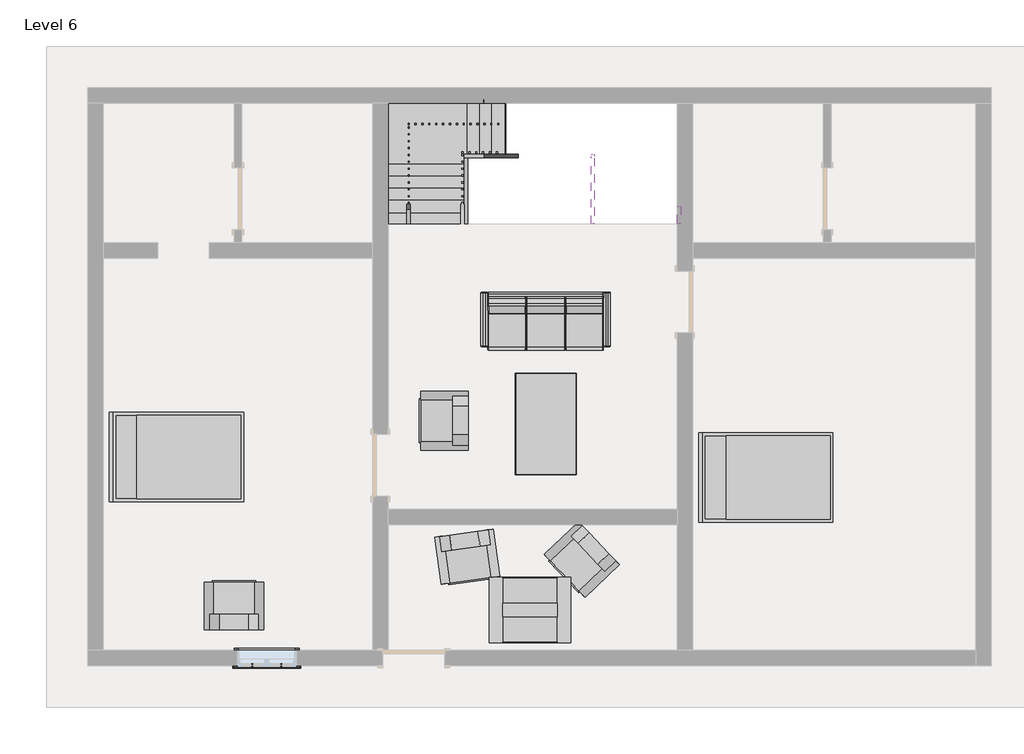
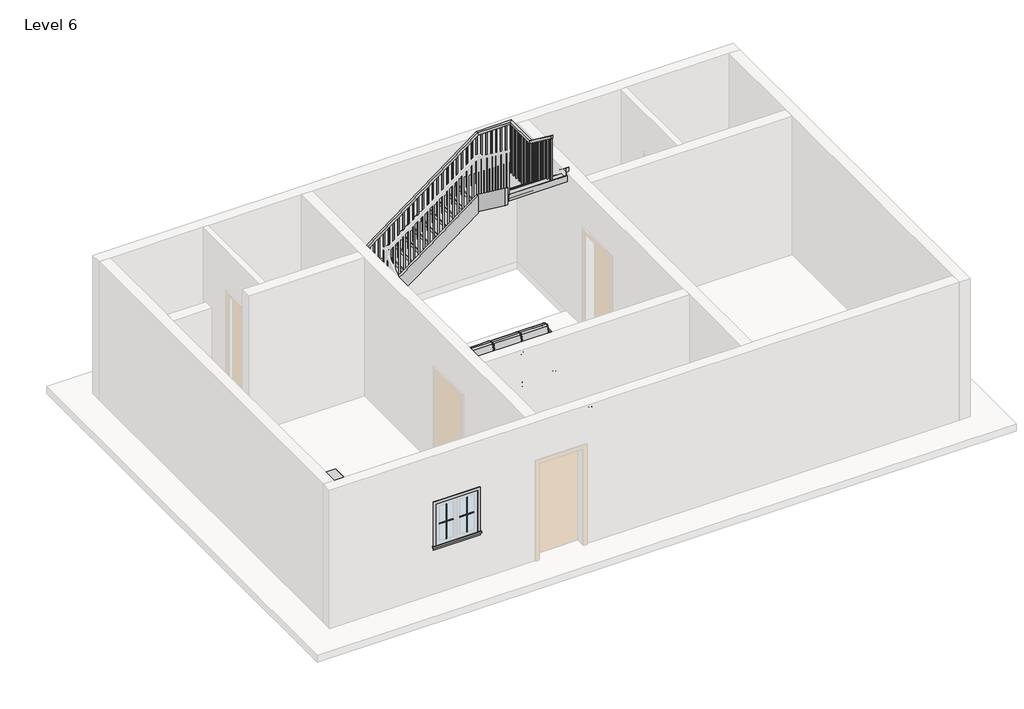
# One storey, part 2 of 2: 9 furniture elements, 6 members, 4 proxies, 1 railing, 1 stair flight.
"""IFC4 building model written with IfcOpenShell, lengths in millimetres."""

from ifc_helpers import new_model, si_unit, frame, origin, place, context, project, spatial, polyline, outline, extrude, faceted_brep, transform, mapped, element, save
from components import muntin_pattern_2x2_muntin_pattern_2x2_b3fe6957, muntin_pattern_2x2_muntin_pattern_2x2_3e0ecaf2, trim_window_exterior_flat_with_sill_41619996, trim_window_interior_flat_picture_frame_51c85655, furniture_2fc85b74, furniture_29a9adb8, furniture_57072a26, bed_17739_bed_17739_15c61121, chair_lounge_11461_couch_0866092f, dining_table_14755_dining_table_14755_d89cb775, wood_and_glass_coffee_table_17065_wood_and_glass_coffee_dbc724b2, stair_flight_6a7f422e

model = new_model("IFC4")

# Units and contexts
model_context = context("Model", 3, world=origin())
ifc_project = project(units=[si_unit("LENGTHUNIT", "METRE", prefix="MILLI")], contexts=[model_context])

# Site, building, storey
site = spatial("IfcSite", under=ifc_project)
building = spatial("IfcBuilding", under=site)
storey = spatial("IfcBuildingStorey", under=building, Name="Level 6", Elevation=12801.6)

# Proxies
placement = place(None, origin())
muntin_pattern_2x2_muntin_pattern_2x2_shape = muntin_pattern_2x2_muntin_pattern_2x2_b3fe6957(model_context)
element("IfcBuildingElementProxy", 1, Name="Muntin Pattern_2x2 : Muntin Pattern_2x2", ObjectType="Muntin Pattern_2x2 : Muntin Pattern_2x2", at=placement, inside=storey, context=model_context, shape_type="MappedRepresentation", body=[
    mapped(muntin_pattern_2x2_muntin_pattern_2x2_shape, transform((-5069.3921642, -1799.3582394, 13938.5934313), x_axis=(-1.0, 0.0, 0.0), y_axis=(0.0, -1.0, 0.0), z_axis=(0.0, 0.0, 1.0))),
])
muntin_pattern_2x2_muntin_pattern_2x2_2_shape = muntin_pattern_2x2_muntin_pattern_2x2_3e0ecaf2(model_context)
element("IfcBuildingElementProxy", 2, Name="Muntin Pattern_2x2 : Muntin Pattern_2x2", ObjectType="Muntin Pattern_2x2 : Muntin Pattern_2x2", at=placement, inside=storey, context=model_context, shape_type="MappedRepresentation", body=[
    mapped(muntin_pattern_2x2_muntin_pattern_2x2_2_shape, transform((-5498.0171642, -1799.3582394, 13938.5934313), x_axis=(1.0, 0.0, 0.0), y_axis=(0.0, 1.0, 0.0), z_axis=(0.0, 0.0, 1.0))),
])
trim_window_exterior_flat_with_sill_shape = trim_window_exterior_flat_with_sill_41619996(model_context)
element("IfcBuildingElementProxy", 3, Name="Trim-Window-Exterior-Flat : with Sill", ObjectType="Trim-Window-Exterior-Flat : with Sill", at=placement, inside=storey, context=model_context, shape_type="MappedRepresentation", body=[
    mapped(trim_window_exterior_flat_with_sill_shape, transform((-5283.7046642, -1808.8832394, 14783.1434313), x_axis=(1.0, 0.0, 0.0), y_axis=(0.0, 0.0, 1.0), z_axis=(0.0, -1.0, 0.0))),
])
trim_window_interior_flat_picture_frame_shape = trim_window_interior_flat_picture_frame_51c85655(model_context)
element("IfcBuildingElementProxy", 4, Name="Trim-Window-Interior-Flat : Picture Frame", ObjectType="Trim-Window-Interior-Flat : Picture Frame", at=placement, inside=storey, context=model_context, shape_type="MappedRepresentation", body=[
    mapped(trim_window_interior_flat_picture_frame_shape, transform((-5283.7046642, -1580.2832394, 14783.1434313), x_axis=(-1.0, 0.0, 0.0), y_axis=(0.0, 0.0, 1.0), z_axis=(0.0, 1.0, 0.0))),
])

# Furniture
furniture_shape = furniture_2fc85b74(model_context)
furniture_2_shape = furniture_29a9adb8(model_context)
furniture_3_shape = furniture_57072a26(model_context)
element("IfcFurniture", 5, at=placement, inside=storey, context=model_context, shape_type="MappedRepresentation", body=[
    mapped(furniture_shape, transform((-1166.392994, 2905.4688314, 12801.6), x_axis=(1.0, 0.0, 0.0), y_axis=(0.0, 1.0, 0.0), z_axis=(0.0, 0.0, 1.0))),
    mapped(furniture_2_shape, transform((-1166.392994, 2905.4688314, 12801.6), x_axis=(1.0, 0.0, 0.0), y_axis=(0.0, 1.0, 0.0), z_axis=(0.0, 0.0, 1.0))),
    mapped(furniture_3_shape, transform((-1166.392994, 2905.4688314, 12801.6), x_axis=(1.0, 0.0, 0.0), y_axis=(0.0, 1.0, 0.0), z_axis=(0.0, 0.0, 1.0))),
])
bed_17739_bed_17739_shape = bed_17739_bed_17739_15c61121(model_context)
element("IfcFurniture", 6, ObjectType="Bed_17739 : Bed_17739", at=placement, inside=storey, context=model_context, shape_type="MappedRepresentation", body=[
    mapped(bed_17739_bed_17739_shape, transform((-6591.8046642, 1277.2167606, 12801.6), x_axis=(0.0, 1.0, 0.0), y_axis=(-1.0, 0.0, 0.0), z_axis=(0.0, 0.0, 1.0))),
])
element("IfcFurniture", 7, ObjectType="Bed_17739 : Bed_17739", at=placement, inside=storey, context=model_context, shape_type="MappedRepresentation", body=[
    mapped(bed_17739_bed_17739_shape, transform((2107.6953358, 972.4167606, 12801.6), x_axis=(0.0, 1.0, 0.0), y_axis=(-1.0, 0.0, 0.0), z_axis=(0.0, 0.0, 1.0))),
])
chair_lounge_11461_couch_shape = chair_lounge_11461_couch_0866092f(model_context)
element("IfcFurniture", 8, ObjectType="Chair-Lounge_11461 : Couch", at=placement, inside=storey, context=model_context, shape_type="MappedRepresentation", body=[
    mapped(chair_lounge_11461_couch_shape, transform((-5766.3046642, -1273.9095448, 12801.6), x_axis=(-1.0, 0.0, 0.0), y_axis=(0.0, -1.0, 0.0), z_axis=(0.0, 0.0, 1.0))),
])
element("IfcFurniture", 9, ObjectType="Chair-Lounge_11461 : Couch", at=placement, inside=storey, context=model_context, shape_type="MappedRepresentation", body=[
    mapped(chair_lounge_11461_couch_shape, transform((-2311.9046642, 1810.6167606, 12801.6), x_axis=(0.0, -1.0, 0.0), y_axis=(1.0, 0.0, 0.0), z_axis=(0.0, 0.0, 1.0))),
])
element("IfcFurniture", 10, ObjectType="Chair-Lounge_11461 : Couch", at=placement, inside=storey, context=model_context, shape_type="MappedRepresentation", body=[
    mapped(chair_lounge_11461_couch_shape, transform((-2372.9488995, 149.9169276, 12801.6), x_axis=(0.9905324493396854, 0.1372787922627668, 0.0), y_axis=(-0.1372787922627668, 0.9905324493396854, 0.0), z_axis=(0.0, 0.0, 1.0))),
])
element("IfcFurniture", 11, ObjectType="Chair-Lounge_11461 : Couch", at=placement, inside=storey, context=model_context, shape_type="MappedRepresentation", body=[
    mapped(chair_lounge_11461_couch_shape, transform((-378.7925234, 1.7617886, 12801.6), x_axis=(0.6894995564131732, -0.7242861048688133, 0.0), y_axis=(0.7242861048688133, 0.6894995564131732, 0.0), z_axis=(0.0, 0.0, 1.0))),
])
dining_table_14755_dining_table_14755_shape = dining_table_14755_dining_table_14755_d89cb775(model_context)
element("IfcFurniture", 12, ObjectType="Dining_table_14755 : Dining_table_14755", at=placement, inside=storey, context=model_context, shape_type="MappedRepresentation", body=[
    mapped(dining_table_14755_dining_table_14755_shape, transform((-711.7046642, 1010.5167606, 12801.6), x_axis=(0.0, 1.0, 0.0), y_axis=(-1.0, 0.0, 0.0), z_axis=(0.0, 0.0, 1.0))),
])
wood_and_glass_coffee_table_17065_wood_and_glass_coffee_shape = wood_and_glass_coffee_table_17065_wood_and_glass_coffee_dbc724b2(model_context)
element("IfcFurniture", 13, ObjectType="Wood_and_Glass_Coffee_Table_17065 : Wood_and_Glass_Coffee_Table_17065", at=placement, inside=storey, context=model_context, shape_type="MappedRepresentation", body=[
    mapped(wood_and_glass_coffee_table_17065_wood_and_glass_coffee_shape, transform((-1397.5046642, -983.3832394, 12801.6), x_axis=(1.0, 0.0, 0.0), y_axis=(0.0, 1.0, 0.0), z_axis=(0.0, 0.0, 1.0))),
])

# Members
element("IfcMember", 14, ObjectType="Stringer - 2\" Width", at=placement, inside=storey, context=model_context, shape_type="SweptSolid", body=[
    extrude(outline(polyline([(4718.9167606, 12801.6), (4718.9167606, 12949.2508226), (5113.281957, 12949.2508226), (4911.6463024, 12801.6), (4718.9167606, 12801.6)])), frame((-3543.8046642, 0.0, 0.0), z_axis=(1.0, 0.0, 0.0), x_axis=(0.0, 1.0, 0.0)), (0.0, 0.0, 1.0), 50.8),
])
element("IfcMember", 15, ObjectType="Stringer - 2\" Width", at=placement, inside=storey, context=model_context, shape_type="SweptSolid", body=[
    extrude(outline(polyline([(13962.4387795, -1623.6098785), (14618.3484291, -743.5977653), (14618.3484291, -1253.6320422), (13962.4387795, -2133.6441554), (13962.4387795, -1623.6098785)])), frame((0.0, 6496.9167606, 0.0), z_axis=(0.0, 1.0, 0.0), x_axis=(0.0, 0.0, 1.0)), (0.0, 0.0, 1.0), 50.8),
])
element("IfcMember", 16, ObjectType="Stringer - 2\" Width", at=placement, inside=storey, context=model_context, shape_type="SweptSolid", body=[
    extrude(outline(polyline([(4718.9167606, 15749.6227901), (4718.9167606, 15943.5652405), (4979.1229954, 15749.6227901), (4718.9167606, 15749.6227901)])), frame((774.1953358, 0.0, 0.0), z_axis=(1.0, 0.0, 0.0), x_axis=(0.0, 1.0, 0.0)), (0.0, 0.0, 1.0), 50.8),
])
element("IfcMember", 17, ObjectType="Stringer - 2\" Width", at=placement, inside=storey, context=model_context, shape_type="SweptSolid", body=[
    extrude(outline(polyline([(4718.9167606, 12801.6), (4718.9167606, 13038.2522719), (5695.7536537, 13753.5561753), (5695.7536537, 13375.7747195), (4911.6463024, 12801.6), (4718.9167606, 12801.6)])), frame((-2368.6972892, 0.0, 0.0), z_axis=(1.0, 0.0, 0.0), x_axis=(0.0, 1.0, 0.0)), (0.0, 0.0, 1.0), 50.8),
])
element("IfcMember", 18, ObjectType="Stringer - 2\" Width", at=placement, inside=storey, context=model_context, shape_type="SweptSolid", body=[
    extrude(outline(polyline([(13787.2438971, -2368.6972892), (13412.9738041, -2368.6972892), (13412.9738041, -2360.8087204), (14803.0389392, -495.8046642), (15177.6250342, -495.8046642), (15177.6250342, -503.2692636), (13787.2438971, -2368.6972892)])), frame((0.0, 5695.7536537, 0.0), z_axis=(0.0, 1.0, 0.0), x_axis=(0.0, 0.0, 1.0)), (0.0, 0.0, 1.0), 50.8),
])
element("IfcMember", 19, ObjectType="Stringer - 2\" Width", at=placement, inside=storey, context=model_context, shape_type="SweptSolid", body=[
    extrude(outline(polyline([(5746.5536537, 15177.6250342), (5746.5536537, 14840.9022932), (5688.2891085, 14840.9022932), (4718.9167606, 15563.4155283), (4718.9167606, 15943.5652405), (5746.5536537, 15177.6250342)])), frame((-495.8046642, 0.0, 0.0), z_axis=(1.0, 0.0, 0.0), x_axis=(0.0, 1.0, 0.0)), (0.0, 0.0, 1.0), 50.8),
])

# Railing
element("IfcRailing", 20, ObjectType="Handrail - Rectangular", at=placement, inside=storey, context=model_context, shape_type="SolidModel", body=[
    faceted_brep([(-3213.6046642, 4718.9167606, 13848.5217391), (-3213.6046642, 4718.9167606, 13785.1634439), (-3162.8046642, 4718.9167606, 13785.1634439), (-3162.8046642, 4718.9167606, 13848.5217391), (-3213.6046642, 5555.0306195, 14471.712193), (-3213.6046642, 5571.8796657, 14420.912193), (-3162.8046642, 5571.8796657, 14420.912193), (-3162.8046642, 5555.0306195, 14471.712193), (-3213.6046642, 6217.5167606, 14471.712193), (-3213.6046642, 6217.5167606, 14420.912193), (-3162.8046642, 6166.7167606, 14420.912193), (-3162.8046642, 6166.7167606, 14471.712193), (-2551.1185231, 6217.5167606, 14471.712193), (-2534.269477, 6217.5167606, 14420.912193), (-2534.269477, 6166.7167606, 14420.912193), (-2551.1185231, 6166.7167606, 14471.712193), (-239.7185231, 6217.5167606, 16194.4948017), (-222.869477, 6217.5167606, 16143.6948017), (-222.869477, 6166.7167606, 16143.6948017), (-239.7185231, 6166.7167606, 16194.4948017), (494.7953358, 6217.5167606, 16194.4948017), (494.7953358, 6217.5167606, 16143.6948017), (443.9953358, 6166.7167606, 16143.6948017), (443.9953358, 6166.7167606, 16194.4948017), (494.7953358, 5483.0029017, 16194.4948017), (494.7953358, 5466.1538556, 16143.6948017), (443.9953358, 5466.1538556, 16143.6948017), (443.9953358, 5483.0029017, 16194.4948017), (494.7953358, 4718.9167606, 16764.0), (443.9953358, 4718.9167606, 16764.0), (443.9953358, 4718.9167606, 16700.6417047), (494.7953358, 4718.9167606, 16700.6417047)], [[[0, 1, 2, 3]], [[1, 0, 4, 5]], [[2, 1, 5, 6]], [[3, 2, 6, 7]], [[0, 3, 7, 4]], [[5, 4, 8, 9]], [[6, 5, 9, 10]], [[7, 6, 10, 11]], [[4, 7, 11, 8]], [[9, 8, 12, 13]], [[10, 9, 13, 14]], [[11, 10, 14, 15]], [[8, 11, 15, 12]], [[13, 12, 16, 17]], [[14, 13, 17, 18]], [[15, 14, 18, 19]], [[12, 15, 19, 16]], [[17, 16, 20, 21]], [[18, 17, 21, 22]], [[19, 18, 22, 23]], [[16, 19, 23, 20]], [[21, 20, 24, 25]], [[22, 21, 25, 26]], [[23, 22, 26, 27]], [[20, 23, 27, 24]], [[28, 29, 30, 31]], [[25, 24, 28, 31]], [[26, 25, 31, 30]], [[27, 26, 30, 29]], [[24, 27, 29, 28]]]),
    extrude(outline(polyline([(4779.2417606, 16655.6789718), (4779.2417606, 15717.0782609), (4760.1917606, 15717.0782609), (4760.1917606, 16669.8777296), (4779.2417606, 16655.6789718)])), frame((459.8703358, 0.0, 0.0), z_axis=(1.0, 0.0, 0.0), x_axis=(0.0, 1.0, 0.0)), (0.0, 0.0, 1.0), 19.05),
    extrude(outline(polyline([(4880.8417606, 16579.9522637), (4880.8417606, 15717.0782609), (4861.7917606, 15717.0782609), (4861.7917606, 16594.1510215), (4880.8417606, 16579.9522637)])), frame((459.8703358, 0.0, 0.0), z_axis=(1.0, 0.0, 0.0), x_axis=(0.0, 1.0, 0.0)), (0.0, 0.0, 1.0), 19.05),
    extrude(outline(polyline([(4982.4417606, 16504.2255557), (4982.4417606, 15584.5565217), (4963.3917606, 15584.5565217), (4963.3917606, 16518.4243134), (4982.4417606, 16504.2255557)])), frame((459.8703358, 0.0, 0.0), z_axis=(1.0, 0.0, 0.0), x_axis=(0.0, 1.0, 0.0)), (0.0, 0.0, 1.0), 19.05),
    extrude(outline(polyline([(5084.0417606, 16428.4988476), (5084.0417606, 15584.5565217), (5064.9917606, 15584.5565217), (5064.9917606, 16442.6976054), (5084.0417606, 16428.4988476)])), frame((459.8703358, 0.0, 0.0), z_axis=(1.0, 0.0, 0.0), x_axis=(0.0, 1.0, 0.0)), (0.0, 0.0, 1.0), 19.05),
    extrude(outline(polyline([(5185.6417606, 16352.7721395), (5185.6417606, 15452.0347826), (5166.5917606, 15452.0347826), (5166.5917606, 16366.9708973), (5185.6417606, 16352.7721395)])), frame((459.8703358, 0.0, 0.0), z_axis=(1.0, 0.0, 0.0), x_axis=(0.0, 1.0, 0.0)), (0.0, 0.0, 1.0), 19.05),
    extrude(outline(polyline([(5287.2417606, 16277.0454314), (5287.2417606, 15319.5130435), (5268.1917606, 15319.5130435), (5268.1917606, 16291.2441892), (5287.2417606, 16277.0454314)])), frame((459.8703358, 0.0, 0.0), z_axis=(1.0, 0.0, 0.0), x_axis=(0.0, 1.0, 0.0)), (0.0, 0.0, 1.0), 19.05),
    extrude(outline(polyline([(5388.8417606, 16201.3187234), (5388.8417606, 15319.5130435), (5369.7917606, 15319.5130435), (5369.7917606, 16215.5174811), (5388.8417606, 16201.3187234)])), frame((459.8703358, 0.0, 0.0), z_axis=(1.0, 0.0, 0.0), x_axis=(0.0, 1.0, 0.0)), (0.0, 0.0, 1.0), 19.05),
    extrude(outline(polyline([(5490.4417606, 16125.5920153), (5490.4417606, 15186.9913043), (5471.3917606, 15186.9913043), (5471.3917606, 16139.7907731), (5490.4417606, 16125.5920153)])), frame((459.8703358, 0.0, 0.0), z_axis=(1.0, 0.0, 0.0), x_axis=(0.0, 1.0, 0.0)), (0.0, 0.0, 1.0), 19.05),
    extrude(outline(polyline([(478.9203358, 5592.0417606), (478.9203358, 5572.9917606), (459.8703358, 5572.9917606), (459.8703358, 5592.0417606), (478.9203358, 5592.0417606)])), frame((0.0, 0.0, 15186.9913043), z_axis=(0.0, 0.0, 1.0), x_axis=(1.0, 0.0, 0.0)), (0.0, 0.0, 1.0), 956.7034973),
    extrude(outline(polyline([(478.9203358, 5693.6417606), (478.9203358, 5674.5917606), (459.8703358, 5674.5917606), (459.8703358, 5693.6417606), (478.9203358, 5693.6417606)])), frame((0.0, 0.0, 15054.4695652), z_axis=(0.0, 0.0, 1.0), x_axis=(1.0, 0.0, 0.0)), (0.0, 0.0, 1.0), 1089.2252364),
    extrude(outline(polyline([(478.9203358, 5795.2417606), (478.9203358, 5776.1917606), (459.8703358, 5776.1917606), (459.8703358, 5795.2417606), (478.9203358, 5795.2417606)])), frame((0.0, 0.0, 15054.4695652), z_axis=(0.0, 0.0, 1.0), x_axis=(1.0, 0.0, 0.0)), (0.0, 0.0, 1.0), 1089.2252364),
    extrude(outline(polyline([(478.9203358, 5896.8417606), (478.9203358, 5877.7917606), (459.8703358, 5877.7917606), (459.8703358, 5896.8417606), (478.9203358, 5896.8417606)])), frame((0.0, 0.0, 15054.4695652), z_axis=(0.0, 0.0, 1.0), x_axis=(1.0, 0.0, 0.0)), (0.0, 0.0, 1.0), 1089.2252364),
    extrude(outline(polyline([(478.9203358, 5998.4417606), (478.9203358, 5979.3917606), (459.8703358, 5979.3917606), (459.8703358, 5998.4417606), (478.9203358, 5998.4417606)])), frame((0.0, 0.0, 15054.4695652), z_axis=(0.0, 0.0, 1.0), x_axis=(1.0, 0.0, 0.0)), (0.0, 0.0, 1.0), 1089.2252364),
    extrude(outline(polyline([(478.9203358, 6100.0417606), (478.9203358, 6080.9917606), (459.8703358, 6080.9917606), (459.8703358, 6100.0417606), (478.9203358, 6100.0417606)])), frame((0.0, 0.0, 15054.4695652), z_axis=(0.0, 0.0, 1.0), x_axis=(1.0, 0.0, 0.0)), (0.0, 0.0, 1.0), 1089.2252364),
    extrude(outline(polyline([(358.2703358, 6201.6417606), (377.3203358, 6201.6417606), (377.3203358, 6182.5917606), (358.2703358, 6182.5917606), (358.2703358, 6201.6417606)])), frame((0.0, 0.0, 15054.4695652), z_axis=(0.0, 0.0, 1.0), x_axis=(1.0, 0.0, 0.0)), (0.0, 0.0, 1.0), 1089.2252364),
    extrude(outline(polyline([(256.6703358, 6201.6417606), (275.7203358, 6201.6417606), (275.7203358, 6182.5917606), (256.6703358, 6182.5917606), (256.6703358, 6201.6417606)])), frame((0.0, 0.0, 15054.4695652), z_axis=(0.0, 0.0, 1.0), x_axis=(1.0, 0.0, 0.0)), (0.0, 0.0, 1.0), 1089.2252364),
    extrude(outline(polyline([(155.0703358, 6201.6417606), (174.1203358, 6201.6417606), (174.1203358, 6182.5917606), (155.0703358, 6182.5917606), (155.0703358, 6201.6417606)])), frame((0.0, 0.0, 15054.4695652), z_axis=(0.0, 0.0, 1.0), x_axis=(1.0, 0.0, 0.0)), (0.0, 0.0, 1.0), 1089.2252364),
    extrude(outline(polyline([(53.4703358, 6201.6417606), (72.5203358, 6201.6417606), (72.5203358, 6182.5917606), (53.4703358, 6182.5917606), (53.4703358, 6201.6417606)])), frame((0.0, 0.0, 15054.4695652), z_axis=(0.0, 0.0, 1.0), x_axis=(1.0, 0.0, 0.0)), (0.0, 0.0, 1.0), 1089.2252364),
    extrude(outline(polyline([(-48.1296642, 6201.6417606), (-29.0796642, 6201.6417606), (-29.0796642, 6182.5917606), (-48.1296642, 6182.5917606), (-48.1296642, 6201.6417606)])), frame((0.0, 0.0, 15054.4695652), z_axis=(0.0, 0.0, 1.0), x_axis=(1.0, 0.0, 0.0)), (0.0, 0.0, 1.0), 1089.2252364),
    extrude(outline(polyline([(-149.7296642, 6201.6417606), (-130.6796642, 6201.6417606), (-130.6796642, 6182.5917606), (-149.7296642, 6182.5917606), (-149.7296642, 6201.6417606)])), frame((0.0, 0.0, 15054.4695652), z_axis=(0.0, 0.0, 1.0), x_axis=(1.0, 0.0, 0.0)), (0.0, 0.0, 1.0), 1089.2252364),
    extrude(outline(polyline([(16122.4822397, -251.3296642), (15054.4695652, -251.3296642), (15054.4695652, -232.2796642), (16136.6809975, -232.2796642), (16122.4822397, -251.3296642)])), frame((0.0, 6182.5917606, 0.0), z_axis=(0.0, 1.0, 0.0), x_axis=(0.0, 0.0, 1.0)), (0.0, 0.0, 1.0), 19.05),
    extrude(outline(polyline([(16046.7555316, -352.9296642), (15054.4695652, -352.9296642), (15054.4695652, -333.8796642), (16060.9542894, -333.8796642), (16046.7555316, -352.9296642)])), frame((0.0, 6182.5917606, 0.0), z_axis=(0.0, 1.0, 0.0), x_axis=(0.0, 0.0, 1.0)), (0.0, 0.0, 1.0), 19.05),
    extrude(outline(polyline([(15971.0288236, -454.5296642), (15054.4695652, -454.5296642), (15054.4695652, -435.4796642), (15985.2275813, -435.4796642), (15971.0288236, -454.5296642)])), frame((0.0, 6182.5917606, 0.0), z_axis=(0.0, 1.0, 0.0), x_axis=(0.0, 0.0, 1.0)), (0.0, 0.0, 1.0), 19.05),
    extrude(outline(polyline([(15895.3021155, -556.1296642), (14921.9478261, -556.1296642), (14921.9478261, -537.0796642), (15909.5008733, -537.0796642), (15895.3021155, -556.1296642)])), frame((0.0, 6182.5917606, 0.0), z_axis=(0.0, 1.0, 0.0), x_axis=(0.0, 0.0, 1.0)), (0.0, 0.0, 1.0), 19.05),
    extrude(outline(polyline([(15819.5754074, -657.7296642), (14921.9478261, -657.7296642), (14921.9478261, -638.6796642), (15833.7741652, -638.6796642), (15819.5754074, -657.7296642)])), frame((0.0, 6182.5917606, 0.0), z_axis=(0.0, 1.0, 0.0), x_axis=(0.0, 0.0, 1.0)), (0.0, 0.0, 1.0), 19.05),
    extrude(outline(polyline([(15743.8486993, -759.3296642), (14789.426087, -759.3296642), (14789.426087, -740.2796642), (15758.0474571, -740.2796642), (15743.8486993, -759.3296642)])), frame((0.0, 6182.5917606, 0.0), z_axis=(0.0, 1.0, 0.0), x_axis=(0.0, 0.0, 1.0)), (0.0, 0.0, 1.0), 19.05),
    extrude(outline(polyline([(15668.1219913, -860.9296642), (14789.426087, -860.9296642), (14789.426087, -841.8796642), (15682.320749, -841.8796642), (15668.1219913, -860.9296642)])), frame((0.0, 6182.5917606, 0.0), z_axis=(0.0, 1.0, 0.0), x_axis=(0.0, 0.0, 1.0)), (0.0, 0.0, 1.0), 19.05),
    extrude(outline(polyline([(15592.3952832, -962.5296642), (14656.9043478, -962.5296642), (14656.9043478, -943.4796642), (15606.594041, -943.4796642), (15592.3952832, -962.5296642)])), frame((0.0, 6182.5917606, 0.0), z_axis=(0.0, 1.0, 0.0), x_axis=(0.0, 0.0, 1.0)), (0.0, 0.0, 1.0), 19.05),
    extrude(outline(polyline([(15516.6685751, -1064.1296642), (14656.9043478, -1064.1296642), (14656.9043478, -1045.0796642), (15530.8673329, -1045.0796642), (15516.6685751, -1064.1296642)])), frame((0.0, 6182.5917606, 0.0), z_axis=(0.0, 1.0, 0.0), x_axis=(0.0, 0.0, 1.0)), (0.0, 0.0, 1.0), 19.05),
    extrude(outline(polyline([(15440.941867, -1165.7296642), (14524.3826087, -1165.7296642), (14524.3826087, -1146.6796642), (15455.1406248, -1146.6796642), (15440.941867, -1165.7296642)])), frame((0.0, 6182.5917606, 0.0), z_axis=(0.0, 1.0, 0.0), x_axis=(0.0, 0.0, 1.0)), (0.0, 0.0, 1.0), 19.05),
    extrude(outline(polyline([(15365.215159, -1267.3296642), (14391.8608696, -1267.3296642), (14391.8608696, -1248.2796642), (15379.4139167, -1248.2796642), (15365.215159, -1267.3296642)])), frame((0.0, 6182.5917606, 0.0), z_axis=(0.0, 1.0, 0.0), x_axis=(0.0, 0.0, 1.0)), (0.0, 0.0, 1.0), 19.05),
    extrude(outline(polyline([(15289.4884509, -1368.9296642), (14391.8608696, -1368.9296642), (14391.8608696, -1349.8796642), (15303.6872087, -1349.8796642), (15289.4884509, -1368.9296642)])), frame((0.0, 6182.5917606, 0.0), z_axis=(0.0, 1.0, 0.0), x_axis=(0.0, 0.0, 1.0)), (0.0, 0.0, 1.0), 19.05),
    extrude(outline(polyline([(15213.7617428, -1470.5296642), (14259.3391304, -1470.5296642), (14259.3391304, -1451.4796642), (15227.9605006, -1451.4796642), (15213.7617428, -1470.5296642)])), frame((0.0, 6182.5917606, 0.0), z_axis=(0.0, 1.0, 0.0), x_axis=(0.0, 0.0, 1.0)), (0.0, 0.0, 1.0), 19.05),
    extrude(outline(polyline([(15138.0350347, -1572.1296642), (14259.3391304, -1572.1296642), (14259.3391304, -1553.0796642), (15152.2337925, -1553.0796642), (15138.0350347, -1572.1296642)])), frame((0.0, 6182.5917606, 0.0), z_axis=(0.0, 1.0, 0.0), x_axis=(0.0, 0.0, 1.0)), (0.0, 0.0, 1.0), 19.05),
    extrude(outline(polyline([(15062.3083267, -1673.7296642), (14126.8173913, -1673.7296642), (14126.8173913, -1654.6796642), (15076.5070844, -1654.6796642), (15062.3083267, -1673.7296642)])), frame((0.0, 6182.5917606, 0.0), z_axis=(0.0, 1.0, 0.0), x_axis=(0.0, 0.0, 1.0)), (0.0, 0.0, 1.0), 19.05),
    extrude(outline(polyline([(14986.5816186, -1775.3296642), (14126.8173913, -1775.3296642), (14126.8173913, -1756.2796642), (15000.7803764, -1756.2796642), (14986.5816186, -1775.3296642)])), frame((0.0, 6182.5917606, 0.0), z_axis=(0.0, 1.0, 0.0), x_axis=(0.0, 0.0, 1.0)), (0.0, 0.0, 1.0), 19.05),
    extrude(outline(polyline([(14910.8549105, -1876.9296642), (13994.2956522, -1876.9296642), (13994.2956522, -1857.8796642), (14925.0536683, -1857.8796642), (14910.8549105, -1876.9296642)])), frame((0.0, 6182.5917606, 0.0), z_axis=(0.0, 1.0, 0.0), x_axis=(0.0, 0.0, 1.0)), (0.0, 0.0, 1.0), 19.05),
    extrude(outline(polyline([(14835.1282025, -1978.5296642), (13861.773913, -1978.5296642), (13861.773913, -1959.4796642), (14849.3269602, -1959.4796642), (14835.1282025, -1978.5296642)])), frame((0.0, 6182.5917606, 0.0), z_axis=(0.0, 1.0, 0.0), x_axis=(0.0, 0.0, 1.0)), (0.0, 0.0, 1.0), 19.05),
    extrude(outline(polyline([(14759.4014944, -2080.1296642), (13861.773913, -2080.1296642), (13861.773913, -2061.0796642), (14773.6002521, -2061.0796642), (14759.4014944, -2080.1296642)])), frame((0.0, 6182.5917606, 0.0), z_axis=(0.0, 1.0, 0.0), x_axis=(0.0, 0.0, 1.0)), (0.0, 0.0, 1.0), 19.05),
    extrude(outline(polyline([(14683.6747863, -2181.7296642), (13729.2521739, -2181.7296642), (13729.2521739, -2162.6796642), (14697.8735441, -2162.6796642), (14683.6747863, -2181.7296642)])), frame((0.0, 6182.5917606, 0.0), z_axis=(0.0, 1.0, 0.0), x_axis=(0.0, 0.0, 1.0)), (0.0, 0.0, 1.0), 19.05),
    extrude(outline(polyline([(14607.9480782, -2283.3296642), (13729.2521739, -2283.3296642), (13729.2521739, -2264.2796642), (14622.146836, -2264.2796642), (14607.9480782, -2283.3296642)])), frame((0.0, 6182.5917606, 0.0), z_axis=(0.0, 1.0, 0.0), x_axis=(0.0, 0.0, 1.0)), (0.0, 0.0, 1.0), 19.05),
    extrude(outline(polyline([(14532.2213702, -2384.9296642), (13596.7304348, -2384.9296642), (13596.7304348, -2365.8796642), (14546.4201279, -2365.8796642), (14532.2213702, -2384.9296642)])), frame((0.0, 6182.5917606, 0.0), z_axis=(0.0, 1.0, 0.0), x_axis=(0.0, 0.0, 1.0)), (0.0, 0.0, 1.0), 19.05),
    extrude(outline(polyline([(14456.4946621, -2486.5296642), (13596.7304348, -2486.5296642), (13596.7304348, -2467.4796642), (14470.6934198, -2467.4796642), (14456.4946621, -2486.5296642)])), frame((0.0, 6182.5917606, 0.0), z_axis=(0.0, 1.0, 0.0), x_axis=(0.0, 0.0, 1.0)), (0.0, 0.0, 1.0), 19.05),
    extrude(outline(polyline([(-2588.1296642, 6201.6417606), (-2569.0796642, 6201.6417606), (-2569.0796642, 6182.5917606), (-2588.1296642, 6182.5917606), (-2588.1296642, 6201.6417606)])), frame((0.0, 0.0, 13596.7304348), z_axis=(0.0, 0.0, 1.0), x_axis=(1.0, 0.0, 0.0)), (0.0, 0.0, 1.0), 824.1817582),
    extrude(outline(polyline([(-2689.7296642, 6201.6417606), (-2670.6796642, 6201.6417606), (-2670.6796642, 6182.5917606), (-2689.7296642, 6182.5917606), (-2689.7296642, 6201.6417606)])), frame((0.0, 0.0, 13596.7304348), z_axis=(0.0, 0.0, 1.0), x_axis=(1.0, 0.0, 0.0)), (0.0, 0.0, 1.0), 824.1817582),
    extrude(outline(polyline([(-2791.3296642, 6201.6417606), (-2772.2796642, 6201.6417606), (-2772.2796642, 6182.5917606), (-2791.3296642, 6182.5917606), (-2791.3296642, 6201.6417606)])), frame((0.0, 0.0, 13596.7304348), z_axis=(0.0, 0.0, 1.0), x_axis=(1.0, 0.0, 0.0)), (0.0, 0.0, 1.0), 824.1817582),
    extrude(outline(polyline([(-2892.9296642, 6201.6417606), (-2873.8796642, 6201.6417606), (-2873.8796642, 6182.5917606), (-2892.9296642, 6182.5917606), (-2892.9296642, 6201.6417606)])), frame((0.0, 0.0, 13596.7304348), z_axis=(0.0, 0.0, 1.0), x_axis=(1.0, 0.0, 0.0)), (0.0, 0.0, 1.0), 824.1817582),
    extrude(outline(polyline([(-2994.5296642, 6201.6417606), (-2975.4796642, 6201.6417606), (-2975.4796642, 6182.5917606), (-2994.5296642, 6182.5917606), (-2994.5296642, 6201.6417606)])), frame((0.0, 0.0, 13596.7304348), z_axis=(0.0, 0.0, 1.0), x_axis=(1.0, 0.0, 0.0)), (0.0, 0.0, 1.0), 824.1817582),
    extrude(outline(polyline([(-3096.1296642, 6201.6417606), (-3077.0796642, 6201.6417606), (-3077.0796642, 6182.5917606), (-3096.1296642, 6182.5917606), (-3096.1296642, 6201.6417606)])), frame((0.0, 0.0, 13596.7304348), z_axis=(0.0, 0.0, 1.0), x_axis=(1.0, 0.0, 0.0)), (0.0, 0.0, 1.0), 824.1817582),
    extrude(outline(polyline([(-3197.7296642, 6131.7917606), (-3197.7296642, 6150.8417606), (-3178.6796642, 6150.8417606), (-3178.6796642, 6131.7917606), (-3197.7296642, 6131.7917606)])), frame((0.0, 0.0, 13596.7304348), z_axis=(0.0, 0.0, 1.0), x_axis=(1.0, 0.0, 0.0)), (0.0, 0.0, 1.0), 824.1817582),
    extrude(outline(polyline([(-3197.7296642, 6030.1917606), (-3197.7296642, 6049.2417606), (-3178.6796642, 6049.2417606), (-3178.6796642, 6030.1917606), (-3197.7296642, 6030.1917606)])), frame((0.0, 0.0, 13596.7304348), z_axis=(0.0, 0.0, 1.0), x_axis=(1.0, 0.0, 0.0)), (0.0, 0.0, 1.0), 824.1817582),
    extrude(outline(polyline([(-3197.7296642, 5928.5917606), (-3197.7296642, 5947.6417606), (-3178.6796642, 5947.6417606), (-3178.6796642, 5928.5917606), (-3197.7296642, 5928.5917606)])), frame((0.0, 0.0, 13596.7304348), z_axis=(0.0, 0.0, 1.0), x_axis=(1.0, 0.0, 0.0)), (0.0, 0.0, 1.0), 824.1817582),
    extrude(outline(polyline([(-3197.7296642, 5826.9917606), (-3197.7296642, 5846.0417606), (-3178.6796642, 5846.0417606), (-3178.6796642, 5826.9917606), (-3197.7296642, 5826.9917606)])), frame((0.0, 0.0, 13596.7304348), z_axis=(0.0, 0.0, 1.0), x_axis=(1.0, 0.0, 0.0)), (0.0, 0.0, 1.0), 824.1817582),
    extrude(outline(polyline([(-3197.7296642, 5725.3917606), (-3197.7296642, 5744.4417606), (-3178.6796642, 5744.4417606), (-3178.6796642, 5725.3917606), (-3197.7296642, 5725.3917606)])), frame((0.0, 0.0, 13596.7304348), z_axis=(0.0, 0.0, 1.0), x_axis=(1.0, 0.0, 0.0)), (0.0, 0.0, 1.0), 824.1817582),
    extrude(outline(polyline([(-3197.7296642, 5623.7917606), (-3197.7296642, 5642.8417606), (-3178.6796642, 5642.8417606), (-3178.6796642, 5623.7917606), (-3197.7296642, 5623.7917606)])), frame((0.0, 0.0, 13596.7304348), z_axis=(0.0, 0.0, 1.0), x_axis=(1.0, 0.0, 0.0)), (0.0, 0.0, 1.0), 824.1817582),
    extrude(outline(polyline([(5541.2417606, 14398.0764873), (5541.2417606, 13464.2086957), (5522.1917606, 13464.2086957), (5522.1917606, 14383.8777296), (5541.2417606, 14398.0764873)])), frame((-3197.7296642, 0.0, 0.0), z_axis=(1.0, 0.0, 0.0), x_axis=(0.0, 1.0, 0.0)), (0.0, 0.0, 1.0), 19.05),
    extrude(outline(polyline([(5439.6417606, 14322.3497793), (5439.6417606, 13464.2086957), (5420.5917606, 13464.2086957), (5420.5917606, 14308.1510215), (5439.6417606, 14322.3497793)])), frame((-3197.7296642, 0.0, 0.0), z_axis=(1.0, 0.0, 0.0), x_axis=(0.0, 1.0, 0.0)), (0.0, 0.0, 1.0), 19.05),
    extrude(outline(polyline([(5338.0417606, 14246.6230712), (5338.0417606, 13331.6869565), (5318.9917606, 13331.6869565), (5318.9917606, 14232.4243134), (5338.0417606, 14246.6230712)])), frame((-3197.7296642, 0.0, 0.0), z_axis=(1.0, 0.0, 0.0), x_axis=(0.0, 1.0, 0.0)), (0.0, 0.0, 1.0), 19.05),
    extrude(outline(polyline([(5236.4417606, 14170.8963631), (5236.4417606, 13199.1652174), (5217.3917606, 13199.1652174), (5217.3917606, 14156.6976054), (5236.4417606, 14170.8963631)])), frame((-3197.7296642, 0.0, 0.0), z_axis=(1.0, 0.0, 0.0), x_axis=(0.0, 1.0, 0.0)), (0.0, 0.0, 1.0), 19.05),
    extrude(outline(polyline([(5134.8417606, 14095.169655), (5134.8417606, 13199.1652174), (5115.7917606, 13199.1652174), (5115.7917606, 14080.9708973), (5134.8417606, 14095.169655)])), frame((-3197.7296642, 0.0, 0.0), z_axis=(1.0, 0.0, 0.0), x_axis=(0.0, 1.0, 0.0)), (0.0, 0.0, 1.0), 19.05),
    extrude(outline(polyline([(5033.2417606, 14019.442947), (5033.2417606, 13066.6434783), (5014.1917606, 13066.6434783), (5014.1917606, 14005.2441892), (5033.2417606, 14019.442947)])), frame((-3197.7296642, 0.0, 0.0), z_axis=(1.0, 0.0, 0.0), x_axis=(0.0, 1.0, 0.0)), (0.0, 0.0, 1.0), 19.05),
    extrude(outline(polyline([(4931.6417606, 13943.7162389), (4931.6417606, 13066.6434783), (4912.5917606, 13066.6434783), (4912.5917606, 13929.5174811), (4931.6417606, 13943.7162389)])), frame((-3197.7296642, 0.0, 0.0), z_axis=(1.0, 0.0, 0.0), x_axis=(0.0, 1.0, 0.0)), (0.0, 0.0, 1.0), 19.05),
    extrude(outline(polyline([(4830.0417606, 13867.9895308), (4830.0417606, 12934.1217391), (4810.9917606, 12934.1217391), (4810.9917606, 13853.7907731), (4830.0417606, 13867.9895308)])), frame((-3197.7296642, 0.0, 0.0), z_axis=(1.0, 0.0, 0.0), x_axis=(0.0, 1.0, 0.0)), (0.0, 0.0, 1.0), 19.05),
    extrude(outline(polyline([(459.8703358, 6201.6417606), (478.9203358, 6201.6417606), (478.9203358, 6182.5917606), (459.8703358, 6182.5917606), (459.8703358, 6201.6417606)])), frame((0.0, 0.0, 15054.4695652), z_axis=(0.0, 0.0, 1.0), x_axis=(1.0, 0.0, 0.0)), (0.0, 0.0, 1.0), 1089.2252364),
    extrude(outline(polyline([(-3197.7296642, 6182.5917606), (-3197.7296642, 6201.6417606), (-3178.6796642, 6201.6417606), (-3178.6796642, 6182.5917606), (-3197.7296642, 6182.5917606)])), frame((0.0, 0.0, 13596.7304348), z_axis=(0.0, 0.0, 1.0), x_axis=(1.0, 0.0, 0.0)), (0.0, 0.0, 1.0), 824.1817582),
    extrude(outline(polyline([(4737.9667606, 16686.442947), (4737.9667606, 15717.0782609), (4718.9167606, 15717.0782609), (4718.9167606, 16700.6417047), (4737.9667606, 16686.442947)])), frame((459.8703358, 0.0, 0.0), z_axis=(1.0, 0.0, 0.0), x_axis=(0.0, 1.0, 0.0)), (0.0, 0.0, 1.0), 19.05),
    extrude(outline(polyline([(4737.9667606, 13799.3622016), (4737.9667606, 12934.1217391), (4718.9167606, 12934.1217391), (4718.9167606, 13785.1634439), (4737.9667606, 13799.3622016)])), frame((-3197.7296642, 0.0, 0.0), z_axis=(1.0, 0.0, 0.0), x_axis=(0.0, 1.0, 0.0)), (0.0, 0.0, 1.0), 19.05),
])

# Stair flight
stair_flight_shape = stair_flight_6a7f422e(model_context)
element("IfcStairFlight", 21, ObjectType="2\" Tread 1\" Nosing 1/4\" Riser", at=placement, inside=storey, context=model_context, shape_type="MappedRepresentation", body=[
    mapped(stair_flight_shape, transform((0.0, 0.0, 0.0), x_axis=(1.0, 0.0, 0.0), y_axis=(0.0, 1.0, 0.0), z_axis=(0.0, 0.0, 1.0))),
])

save(model, "model.ifc")

# Revit data of these elements
# Type "Muntin Pattern_2x2 : Muntin Pattern_2x2"
#   Width [instance default] = 4' - 0"
#   Thickness = 0' - 0 1/2"
#   Height [instance default] = 4' - 0"
#   Distance = 0' - 0 3/4"
#   Interior Material [instance default] = none
#   Exterior Material [instance default] = none
#   Default Elevation = 0
# Type "Trim-Window-Exterior-Flat : with Sill"
#   Trim Width = 0' - 2 1/4"
#   Trim Thickness_Picture Frame = 0' - 1 1/4"
#   Trim Thickness_with Sill = 0' - 0 3/4"
#   Sill Thickness = 0' - 1 1/4"
#   Opening Width [instance default] = 2' - 0"
#   Opening Height [instance default] = 3' - 0"
#   Default Elevation = 4' - 0"
#   Sill = yes
#   Picture Frame = no
#   Trim Material [instance default] = none
# Type "Trim-Window-Interior-Flat : Picture Frame"
#   Trim Thickness_Picture Frame = 0' - 1 1/4"
#   Trim Width = 0' - 2 1/4"
#   Trim Thickness_with Sill = 0' - 0 3/4"
#   Sill Thickness = 0' - 1 1/4"
#   Opening Width [instance default] = 2' - 0"
#   Opening Height [instance default] = 3' - 0"
#   Default Elevation = 4' - 0"
#   Sill = no
#   Picture Frame = yes
#   Trim Material [instance default] = none
# Type
#   Width [instance] = 6' - 3.19685"
#   Default Elevation = 0
# Type "Bed_17739 : Bed_17739"
#   Default Elevation = 0
# Type "Chair-Lounge_11461 : Couch"
#   Default Elevation = 0
#   Assembly Code = ""
# Type "Dining_table_14755 : Dining_table_14755"
#   Lengte [instance default] = 4' - 11.05512"
#   Breedte [instance default] = 2' - 11.43307"
#   Tafelblad = none
#   Poten = none
#   Default Elevation = 0
# Type "Wood_and_Glass_Coffee_Table_17065 : Wood_and_Glass_Coffee_Table_17065"
#   Coffee Table Wood Width = 0' - 7.87402"
#   Coffee Table Width = 3' - 2.17592"
#   Coffee Table Length = 3' - 11.24409"
#   Wood and Glass Coffee Table - Wood = Wood and Glass Coffee Table - Wood
#   Wood and Glass Coffee Table - Glass = Wood and Glass Coffee Table - Glass
#   Default Elevation = 0
# Type "Handrail - Rectangular"
#   Assembly Code = "C2010400"
#   built-in parameter 1008612 = 0.0416667 (stored number, unit not read)
#   built-in parameter 1008611 = 0.0416667 (stored number, unit not read)
#   built-in parameter 1008609 = 0.333333 (stored number, unit not read)
#   built-in parameter 1008604 = 0.166667 (stored number, unit not read)
#   built-in parameter 1008603 = 0.166667 (stored number, unit not read)
#   Railing Height = 3' - 0"
#   built-in parameter 1008630 = 2
#   built-in parameter 1008610 = 2
#   built-in parameter 1008618 = Baluster - Square : 3/4"
# Elements 1, 2 (IfcBuildingElementProxy, "Muntin Pattern_2x2 : Muntin Pattern_2x2")
#   Width = 0' - 11 5/8"
#   Height = 2' - 6 1/2"
#   Interior Material = Wood - Stained
#   Exterior Material = Clad - White
#   Phase Created = New Construction
#   Materials on its faces: "Clad - White", "Wood - Stained"
# Element 3 (IfcBuildingElementProxy, "Trim-Window-Exterior-Flat : with Sill")
#   Opening Width = 2' - 10"
#   Opening Height = 3' - 0"
#   Trim Material = Clad - White
#   Phase Created = New Construction
#   Materials on its faces: "Clad - White"
# Element 4 (IfcBuildingElementProxy, "Trim-Window-Interior-Flat : Picture Frame")
#   Opening Width = 2' - 10"
#   Opening Height = 3' - 0"
#   Trim Material = Wood - Stained
#   Phase Created = New Construction
#   Materials on its faces: "Wood - Stained"
# Element 5 (IfcFurniture)
#   Width = 6' - 3.19685"
#   Phase Created = New Construction
# Elements 6, 7 (IfcFurniture, "Bed_17739 : Bed_17739")
#   Phase Created = New Construction
#   Materials on its faces: "legs", "sheets", "bed frame", "Blanket"
# Elements 8, 9, 10, 11 (IfcFurniture, "Chair-Lounge_11461 : Couch")
#   Phase Created = New Construction
# Element 12 (IfcFurniture, "Dining_table_14755 : Dining_table_14755")
#   Lengte = 4' - 11.05512"
#   Breedte = 2' - 11.43307"
#   Phase Created = New Construction
# Element 13 (IfcFurniture, "Wood_and_Glass_Coffee_Table_17065 : Wood_and_Glass_Coffee_Table_17065")
#   Phase Created = New Construction
#   Materials on its faces: "Wood and Glass Coffee Table - Wood", "Wood and Glass Coffee Table - Glass"
# Elements 14, 15, 16, 17, 18, 19 (IfcMember, "Stringer - 2\" Width")
#   Phase Created = New Construction
# Element 20 (IfcRailing, "Handrail - Rectangular")
#   Phase Created = New Construction
# Element 21 (IfcStairFlight, "2\" Tread 1\" Nosing 1/4\" Riser")
#   Phase Created = New Construction
# Materials
#   "Wood and Glass Coffee Table - Wood": class "Generic", colour RGB 120 120 120, transparency 0, Cost = 0
#   "Wood and Glass Coffee Table - Glass": class "Generic", colour RGB 120 120 120, transparency 0, Cost = 0
#   "Clad - White": class "Wood", colour RGB 242 242 238, transparency 0, Cost = 0
#   "Wood - Stained": class "Wood", colour RGB 224 178 126, transparency 0, Cost = 0
#   "legs": colour RGB 90 73 37, transparency 0, Cost = 0
#   "sheets": colour RGB 200 195 176, transparency 0, Cost = 0
#   "bed frame": colour RGB 90 73 37, transparency 0, Cost = 0
#   "Blanket": class "System", colour RGB 59 0 1, transparency 0, Cost = 0
